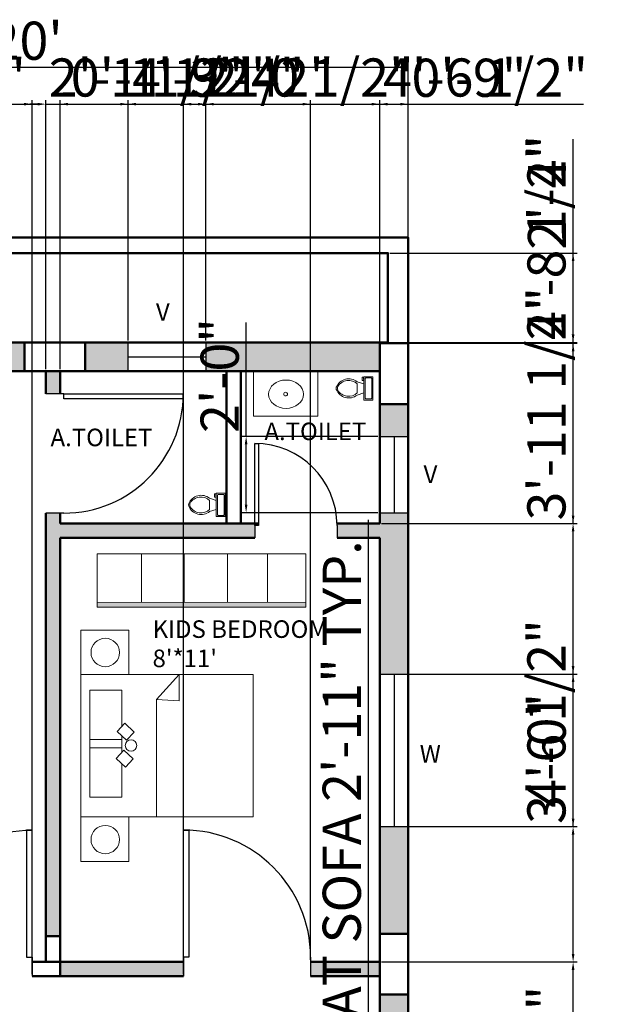
# Model space of a CAD drawing. Units: inches. Extents: x 2063 to 3370, y 2091 to 2971.
# Tile 14 of 14: x 3185 to 3370, y 2623 to 2933. Entities that reach past the tile are written whole.
import ezdxf

# ---------------------------------------------------------------- set-up
doc = ezdxf.new("R2010")
doc.units = ezdxf.units.IN
for name, color, linetype, lineweight in [('A-ANNO-DIMS', 2, 'Continuous', 18), ('A-ANNO-TEXT', 7, 'Continuous', 18), ('A-AREA-IDEN', 3, 'Continuous', 18), ('A-COLS', 7, 'Continuous', 50), ('A-DOOR', 4, 'Continuous', 25), ('A-FLOR-FIXT', 9, 'Continuous', 18), ('A-FURN', 8, 'Continuous', 18), ('A-GLAZ', 131, 'Continuous', 25), ('A-WALL', 7, 'Continuous', 50), ('A-WALL-PATT', 8, 'Continuous', 13)]:
    doc.layers.add(name, color=color, linetype=linetype, lineweight=lineweight)
doc.styles.get("Standard").update_dxf_attribs({"font": 'arial.ttf'})
doc.dimstyles.new('ISO-25', dxfattribs={"dimtxt": 12, "dimasz": 2.5, "dimexe": 1.25, "dimexo": 0.625, "dimtad": 1, "dimdec": 0, "dimlunit": 4, "dimtxsty": 'Standard', "dimcen": 2.5, "dimadec": 0, "dimazin": 0, "dimtfac": 1, "dimtdec": 0, "dimtmove": 0, "dimatfit": 3, "dimfxl": 1, "dimarcsym": 0})

# ---------------------------------------------------------------- blocks, each defined once
blk = doc.blocks.new('*U2')
for p, q in [((0, 0), (0, -6)), ((40, 0), (40, -6))]:
    blk.add_line(p, q)
blk.add_lwpolyline([(0, 0), (0, 40), (1.75, 40), (1.75, 0)], close=True)
blk.add_arc((0, 0), 40, 0, 90)
blk = doc.blocks.new('*U4')
for p, q in [((-10, -8.5), (-8, -8.5)), ((-10, -9.5), (-10, -8.5)), ((-8, -8.5), (-8, -8)), ((-7, -8), (-7, -9.5)), ((-4, -8), (-6, -14)), ((4, -8), (6, -14)), ((9.5, -6), (9.5, -2)), ((-7, -9.5), (-10, -9.5)), ((4, -14), (-4, -14))]:
    blk.add_line(p, q)
blk.add_lwpolyline([(10.5, -8), (10.5, 0), (-10.5, 0), (-10.5, -8)], close=True)
for points in [[(-9.5, -2), (-9.5, -6)], [(8.5, -1), (-8.5, -1)], [(-8.5, -7), (8.5, -7)]]:
    blk.add_lwpolyline(points)
for centre, radius, start, end in [((-8.62, -1.88), 0.884, 81.8699, 188.1301), ((-8.62, -6.12), 0.884, 171.8699, 278.1301), ((8.62, -1.88), 0.884, 351.8699, 98.1301), ((8.62, -6.12), 0.884, 261.8699, 8.1301), ((3.52, -21.58), 12.17, 141.46911, 247.97143), ((4.2, -21.82), 11.33, 136.36773, 238.94682), ((-3.52, -21.58), 12.17, 292.02843, 38.53071), ((-4.2, -21.82), 11.33, 301.05301, 43.63209), ((0, -27.88), 4, 245.73182, 294.26817), ((0, -29), 4, 254.86053, 285.13947)]:
    blk.add_arc(centre, radius, start, end)
blk = doc.blocks.new('*D9')
at = {"layer": 'A-ANNO-DIMS', "color": 0, "lineweight": -2, "transparency": 16777216}
for p, q in [((3067.42, 2865.05), (3067.42, 2919.33)), ((3069.92, 2918.08), (3304.92, 2918.08)), ((3307.42, 2865.05), (3307.42, 2919.33))]:
    blk.add_line(p, q, dxfattribs=at)
at = {"layer": 'A-ANNO-DIMS', "color": 0, "transparency": 16777216}
for points in [[(3069.92, 2918.5), (3069.92, 2917.67), (3067.42, 2918.08)], [(3304.92, 2918.5), (3304.92, 2917.67), (3307.42, 2918.08)]]:
    blk.add_solid(points, dxfattribs=at)
at = {"layer": 'Defpoints', "color": 0, "transparency": 16777216}
for p in [(3307.42, 2918.08), (3067.42, 2864.43), (3307.42, 2864.43)]:
    blk.add_point(p, dxfattribs=at)
at = {"layer": 'A-ANNO-DIMS', "color": 0, "transparency": 16777216, "insert": (3187.42, 2924.84), "char_height": 12, "attachment_point": 5}
blk.add_mtext("20'", dxfattribs=at)
blk = doc.blocks.new('BED-DOUBLE')
for p, q in [((23.79, 50.98), (30.96, 58.78)), ((30.96, 58.78), (30.96, 50.54)), ((23.79, 14), (23.79, 50.98)), ((30.96, 50.54), (23.79, 50.98))]:
    blk.add_line(p, q)
for points in [[(0, 58.78), (15.11, 58.78), (15.11, 72.78), (0, 72.78)], [(0, 58.78), (54.26, 58.78), (54.26, 14), (0, 14)], [(11.45, 40.86), (13.89, 43.46), (16.84, 40.71), (14.4, 38.1)], [(11.16, 32.43), (13.59, 35.03), (16.54, 32.28), (14.11, 29.67)], [(0, 0), (15.11, 0), (15.11, 14), (0, 14)]]:
    blk.add_lwpolyline(points, close=True)
for points in [[(12.88, 42.39), (12.88, 53.87), (2.9, 53.87), (2.9, 35.71), (12.88, 35.71), (12.88, 39.52)], [(12.88, 34.27), (12.88, 38.39), (2.9, 38.39), (2.9, 20.23), (12.88, 20.23), (12.88, 30.81)]]:
    blk.add_lwpolyline(points)
for centre, radius in [((7.71, 65.74), 4.47), ((15.81, 36.46), 1.81), ((7.71, 6.86), 4.47)]:
    blk.add_circle(centre, radius)
blk = doc.blocks.new('WARDROBE')
for p, q in [((13.88, 1.44), (13.88, 16.75)), ((27.33, 1.44), (27.33, 16.75)), ((40.97, 1.44), (40.97, 16.75)), ((53.56, 1.44), (53.56, 16.75)), ((0, 1.42), (65.55, 1.52))]:
    blk.add_line(p, q)
blk.add_lwpolyline([(0, 16.75), (65.55, 16.75), (65.55, 0), (0, 0)], close=True)
blk = doc.blocks.new('*D26')
at = {"layer": 'A-ANNO-DIMS', "color": 0, "lineweight": -2, "transparency": 16777216}
for p, q in [((3294.89, 2575.71), (3294.89, 2775.57)), ((3290.25, 2575.71), (3296.14, 2575.71)), ((3294.89, 2543.09), (3294.89, 2573.21)), ((3290.25, 2540.59), (3296.14, 2540.59))]:
    blk.add_line(p, q, dxfattribs=at)
at = {"layer": 'A-ANNO-DIMS', "color": 0, "transparency": 16777216}
for points in [[(3294.47, 2573.21), (3295.31, 2573.21), (3294.89, 2575.71)], [(3294.47, 2543.09), (3295.31, 2543.09), (3294.89, 2540.59)]]:
    blk.add_solid(points, dxfattribs=at)
at = {"layer": 'Defpoints', "color": 0, "transparency": 16777216}
for p in [(3289.62, 2575.71), (3294.89, 2575.71), (3289.62, 2540.59)]:
    blk.add_point(p, dxfattribs=at)
at = {"layer": 'A-ANNO-DIMS', "color": 0, "transparency": 16777216, "insert": (3288.05, 2676.89), "char_height": 12, "attachment_point": 5, "rotation": 90}
blk.add_mtext('3-SEAT SOFA 2\'-11" TYP.', dxfattribs=at)
blk = doc.blocks.new('*D138')
at = {"layer": 'A-ANNO-DIMS', "color": 0, "lineweight": -2, "transparency": 16777216}
for p, q in [((3167.94, 2832.05), (3167.94, 2907.68)), ((3193.42, 2823.05), (3193.42, 2907.68)), ((3170.44, 2906.43), (3190.92, 2906.43)), ((3193.42, 2906.43), (3257.23, 2906.43))]:
    blk.add_line(p, q, dxfattribs=at)
at = {"layer": 'A-ANNO-DIMS', "color": 0, "transparency": 16777216}
for points in [[(3170.44, 2906.84), (3170.44, 2906.01), (3167.94, 2906.43)], [(3190.92, 2906.84), (3190.92, 2906.01), (3193.42, 2906.43)]]:
    blk.add_solid(points, dxfattribs=at)
at = {"layer": 'Defpoints', "color": 0, "transparency": 16777216}
for p in [(3193.42, 2906.43), (3167.94, 2831.43), (3193.42, 2822.43)]:
    blk.add_point(p, dxfattribs=at)
at = {"layer": 'A-ANNO-DIMS', "color": 0, "transparency": 16777216, "insert": (3226.57, 2913.26), "char_height": 12, "attachment_point": 5}
blk.add_mtext('2\'-1 1/2"', dxfattribs=at)
blk = doc.blocks.new('*D139')
at = {"layer": 'A-ANNO-DIMS', "color": 0, "lineweight": -2, "transparency": 16777216}
for p, q in [((3193.42, 2823.05), (3193.42, 2907.68)), ((3197.92, 2823.05), (3197.92, 2907.68)), ((3190.92, 2906.43), (3188.42, 2906.43)), ((3193.42, 2906.43), (3197.92, 2906.43)), ((3200.42, 2906.43), (3264.03, 2906.43))]:
    blk.add_line(p, q, dxfattribs=at)
at = {"layer": 'A-ANNO-DIMS', "color": 0, "transparency": 16777216}
for points in [[(3190.92, 2906.84), (3190.92, 2906.01), (3193.42, 2906.43)], [(3200.42, 2906.84), (3200.42, 2906.01), (3197.92, 2906.43)]]:
    blk.add_solid(points, dxfattribs=at)
at = {"layer": 'Defpoints', "color": 0, "transparency": 16777216}
for p in [(3197.92, 2906.43), (3193.42, 2822.43), (3197.92, 2822.43)]:
    blk.add_point(p, dxfattribs=at)
at = {"layer": 'A-ANNO-DIMS', "color": 0, "transparency": 16777216, "insert": (3233.47, 2913.26), "char_height": 12, "attachment_point": 5}
blk.add_mtext('0\'-4 1/2"', dxfattribs=at)
blk = doc.blocks.new('*D140')
at = {"layer": 'A-ANNO-DIMS', "color": 0, "lineweight": -2, "transparency": 16777216}
for p, q in [((3197.92, 2823.05), (3197.92, 2907.68)), ((3219.33, 2832.05), (3219.33, 2907.68)), ((3200.42, 2906.43), (3216.83, 2906.43)), ((3219.33, 2906.43), (3281.81, 2906.43))]:
    blk.add_line(p, q, dxfattribs=at)
at = {"layer": 'A-ANNO-DIMS', "color": 0, "transparency": 16777216}
for points in [[(3200.42, 2906.84), (3200.42, 2906.01), (3197.92, 2906.43)], [(3216.83, 2906.84), (3216.83, 2906.01), (3219.33, 2906.43)]]:
    blk.add_solid(points, dxfattribs=at)
at = {"layer": 'Defpoints', "color": 0, "transparency": 16777216}
for p in [(3219.33, 2906.43), (3219.33, 2831.43), (3197.92, 2822.43)]:
    blk.add_point(p, dxfattribs=at)
at = {"layer": 'A-ANNO-DIMS', "color": 0, "transparency": 16777216, "insert": (3251.82, 2913.26), "char_height": 12, "attachment_point": 5}
blk.add_mtext('1\'-9 1/2"', dxfattribs=at)
blk = doc.blocks.new('*D141')
at = {"layer": 'A-ANNO-DIMS', "color": 0, "lineweight": -2, "transparency": 16777216}
for p, q in [((3219.33, 2832.05), (3219.33, 2907.68)), ((3243.76, 2832.05), (3243.76, 2907.68)), ((3221.83, 2906.43), (3241.26, 2906.43)), ((3243.76, 2906.43), (3307.58, 2906.43))]:
    blk.add_line(p, q, dxfattribs=at)
at = {"layer": 'A-ANNO-DIMS', "color": 0, "transparency": 16777216}
for points in [[(3221.83, 2906.84), (3221.83, 2906.01), (3219.33, 2906.43)], [(3241.26, 2906.84), (3241.26, 2906.01), (3243.76, 2906.43)]]:
    blk.add_solid(points, dxfattribs=at)
at = {"layer": 'Defpoints', "color": 0, "transparency": 16777216}
for p in [(3243.76, 2906.43), (3219.33, 2831.43), (3243.76, 2831.43)]:
    blk.add_point(p, dxfattribs=at)
at = {"layer": 'A-ANNO-DIMS', "color": 0, "transparency": 16777216, "insert": (3276.92, 2913.26), "char_height": 12, "attachment_point": 5}
blk.add_mtext('2\'-0 1/2"', dxfattribs=at)
blk = doc.blocks.new('*D142')
at = {"layer": 'A-ANNO-DIMS', "color": 0, "lineweight": -2, "transparency": 16777216}
for p, q in [((3243.76, 2832.05), (3243.76, 2907.68)), ((3298.42, 2823.05), (3298.42, 2907.68)), ((3246.26, 2906.43), (3295.92, 2906.43)), ((3298.42, 2906.43), (3362.51, 2906.43))]:
    blk.add_line(p, q, dxfattribs=at)
at = {"layer": 'A-ANNO-DIMS', "color": 0, "transparency": 16777216}
for points in [[(3246.26, 2906.84), (3246.26, 2906.01), (3243.76, 2906.43)], [(3295.92, 2906.84), (3295.92, 2906.01), (3298.42, 2906.43)]]:
    blk.add_solid(points, dxfattribs=at)
at = {"layer": 'Defpoints', "color": 0, "transparency": 16777216}
for p in [(3298.42, 2906.43), (3243.76, 2831.43), (3298.42, 2822.43)]:
    blk.add_point(p, dxfattribs=at)
at = {"layer": 'A-ANNO-DIMS', "color": 0, "transparency": 16777216, "insert": (3331.71, 2913.26), "char_height": 12, "attachment_point": 5}
blk.add_mtext('4\'-6 1/2"', dxfattribs=at)
blk = doc.blocks.new('*D143')
at = {"layer": 'A-ANNO-DIMS', "color": 0, "lineweight": -2, "transparency": 16777216}
for p, q in [((3298.42, 2823.05), (3298.42, 2907.68)), ((3307.42, 2831.77), (3307.42, 2907.68)), ((3300.92, 2906.43), (3304.92, 2906.43)), ((3307.42, 2906.43), (3343.06, 2906.43))]:
    blk.add_line(p, q, dxfattribs=at)
at = {"layer": 'A-ANNO-DIMS', "color": 0, "transparency": 16777216}
for points in [[(3300.92, 2906.84), (3300.92, 2906.01), (3298.42, 2906.43)], [(3304.92, 2906.84), (3304.92, 2906.01), (3307.42, 2906.43)]]:
    blk.add_solid(points, dxfattribs=at)
at = {"layer": 'Defpoints', "color": 0, "transparency": 16777216}
for p in [(3307.42, 2906.43), (3307.42, 2831.15), (3298.42, 2822.43)]:
    blk.add_point(p, dxfattribs=at)
at = {"layer": 'A-ANNO-DIMS', "color": 0, "transparency": 16777216, "insert": (3326.49, 2913.18), "char_height": 12, "attachment_point": 5}
blk.add_mtext('0\'-9"', dxfattribs=at)
blk = doc.blocks.new('*D164')
at = {"layer": 'A-ANNO-DIMS', "color": 0, "lineweight": -2, "transparency": 16777216}
for p, q in [((3299.04, 2636.43), (3360.49, 2636.43)), ((3359.24, 2587.78), (3359.24, 2633.93)), ((3299.04, 2585.28), (3360.49, 2585.28))]:
    blk.add_line(p, q, dxfattribs=at)
at = {"layer": 'A-ANNO-DIMS', "color": 0, "transparency": 16777216}
for points in [[(3358.82, 2633.93), (3359.66, 2633.93), (3359.24, 2636.43)], [(3358.82, 2587.78), (3359.66, 2587.78), (3359.24, 2585.28)]]:
    blk.add_solid(points, dxfattribs=at)
at = {"layer": 'Defpoints', "color": 0, "transparency": 16777216}
for p in [(3298.42, 2636.43), (3359.24, 2636.43), (3298.42, 2585.28)]:
    blk.add_point(p, dxfattribs=at)
at = {"layer": 'A-ANNO-DIMS', "color": 0, "transparency": 16777216, "insert": (3352.48, 2610.85), "char_height": 12, "attachment_point": 5, "rotation": 90}
blk.add_mtext('4\'-3"', dxfattribs=at)
blk = doc.blocks.new('*D165')
at = {"layer": 'A-ANNO-DIMS', "color": 0, "lineweight": -2, "transparency": 16777216}
for p, q in [((3359.24, 2679.03), (3359.24, 2742.63)), ((3299.04, 2679.03), (3360.49, 2679.03)), ((3359.24, 2638.93), (3359.24, 2676.53)), ((3299.04, 2636.43), (3360.49, 2636.43))]:
    blk.add_line(p, q, dxfattribs=at)
at = {"layer": 'A-ANNO-DIMS', "color": 0, "transparency": 16777216}
for points in [[(3358.82, 2676.53), (3359.66, 2676.53), (3359.24, 2679.03)], [(3358.82, 2638.93), (3359.66, 2638.93), (3359.24, 2636.43)]]:
    blk.add_solid(points, dxfattribs=at)
at = {"layer": 'Defpoints', "color": 0, "transparency": 16777216}
for p in [(3298.42, 2679.03), (3359.24, 2679.03), (3298.42, 2636.43)]:
    blk.add_point(p, dxfattribs=at)
at = {"layer": 'A-ANNO-DIMS', "color": 0, "transparency": 16777216, "insert": (3352.41, 2712.08), "char_height": 12, "attachment_point": 5, "rotation": 90}
blk.add_mtext('3\'-6 1/2"', dxfattribs=at)
blk = doc.blocks.new('*D166')
at = {"layer": 'A-ANNO-DIMS', "color": 0, "lineweight": -2, "transparency": 16777216}
for p, q in [((3299.04, 2727.03), (3360.49, 2727.03)), ((3359.24, 2681.53), (3359.24, 2724.53)), ((3299.04, 2679.03), (3360.49, 2679.03))]:
    blk.add_line(p, q, dxfattribs=at)
at = {"layer": 'A-ANNO-DIMS', "color": 0, "transparency": 16777216}
for points in [[(3358.82, 2724.53), (3359.66, 2724.53), (3359.24, 2727.03)], [(3358.82, 2681.53), (3359.66, 2681.53), (3359.24, 2679.03)]]:
    blk.add_solid(points, dxfattribs=at)
at = {"layer": 'Defpoints', "color": 0, "transparency": 16777216}
for p in [(3298.42, 2727.03), (3359.24, 2727.03), (3298.42, 2679.03)]:
    blk.add_point(p, dxfattribs=at)
at = {"layer": 'A-ANNO-DIMS', "color": 0, "transparency": 16777216, "insert": (3352.49, 2703.03), "char_height": 12, "attachment_point": 5, "rotation": 90}
blk.add_mtext('4\'-0"', dxfattribs=at)
blk = doc.blocks.new('*D167')
at = {"layer": 'A-ANNO-DIMS', "color": 0, "lineweight": -2, "transparency": 16777216}
for p, q in [((3359.24, 2774.43), (3359.24, 2847.35)), ((3299.04, 2774.43), (3360.49, 2774.43)), ((3359.24, 2729.53), (3359.24, 2771.93)), ((3299.04, 2727.03), (3360.49, 2727.03))]:
    blk.add_line(p, q, dxfattribs=at)
at = {"layer": 'A-ANNO-DIMS', "color": 0, "transparency": 16777216}
for points in [[(3358.82, 2771.93), (3359.66, 2771.93), (3359.24, 2774.43)], [(3358.82, 2729.53), (3359.66, 2729.53), (3359.24, 2727.03)]]:
    blk.add_solid(points, dxfattribs=at)
at = {"layer": 'Defpoints', "color": 0, "transparency": 16777216}
for p in [(3298.42, 2774.43), (3359.24, 2774.43), (3298.42, 2727.03)]:
    blk.add_point(p, dxfattribs=at)
at = {"layer": 'A-ANNO-DIMS', "color": 0, "transparency": 16777216, "insert": (3352.41, 2812.14), "char_height": 12, "attachment_point": 5, "rotation": 90}
blk.add_mtext('3\'-11 1/2"', dxfattribs=at)
blk = doc.blocks.new('*D168')
at = {"layer": 'A-ANNO-DIMS', "color": 0, "lineweight": -2, "transparency": 16777216}
for p, q in [((3359.24, 2831.15), (3359.24, 2895.24)), ((3299.04, 2831.15), (3360.49, 2831.15)), ((3359.24, 2776.93), (3359.24, 2828.65)), ((3299.04, 2774.43), (3360.49, 2774.43))]:
    blk.add_line(p, q, dxfattribs=at)
at = {"layer": 'A-ANNO-DIMS', "color": 0, "transparency": 16777216}
for points in [[(3358.82, 2828.65), (3359.66, 2828.65), (3359.24, 2831.15)], [(3358.82, 2776.93), (3359.66, 2776.93), (3359.24, 2774.43)]]:
    blk.add_solid(points, dxfattribs=at)
at = {"layer": 'Defpoints', "color": 0, "transparency": 16777216}
for p in [(3298.42, 2831.15), (3359.24, 2831.15), (3298.42, 2774.43)]:
    blk.add_point(p, dxfattribs=at)
at = {"layer": 'A-ANNO-DIMS', "color": 0, "transparency": 16777216, "insert": (3352.41, 2864.44), "char_height": 12, "attachment_point": 5, "rotation": 90}
blk.add_mtext('4\'-8 1/2"', dxfattribs=at)
blk = doc.blocks.new('*D169')
at = {"layer": 'A-ANNO-DIMS', "color": 0, "lineweight": -2, "transparency": 16777216}
for p, q in [((3359.24, 2859.54), (3359.24, 2895.4)), ((3301.66, 2859.54), (3360.49, 2859.54)), ((3359.24, 2833.93), (3359.24, 2857.04)), ((3301.66, 2831.43), (3360.49, 2831.43))]:
    blk.add_line(p, q, dxfattribs=at)
at = {"layer": 'A-ANNO-DIMS', "color": 0, "transparency": 16777216}
for points in [[(3358.82, 2857.04), (3359.66, 2857.04), (3359.24, 2859.54)], [(3358.82, 2833.93), (3359.66, 2833.93), (3359.24, 2831.43)]]:
    blk.add_solid(points, dxfattribs=at)
at = {"layer": 'Defpoints', "color": 0, "transparency": 16777216}
for p in [(3301.03, 2859.54), (3359.24, 2859.54), (3301.03, 2831.43)]:
    blk.add_point(p, dxfattribs=at)
at = {"layer": 'A-ANNO-DIMS', "color": 0, "transparency": 16777216, "insert": (3352.59, 2878.72), "char_height": 12, "attachment_point": 5, "rotation": 90}
blk.add_mtext('2\'-4"', dxfattribs=at)
blk = doc.blocks.new('*D170')
at = {"layer": 'A-ANNO-DIMS', "color": 0, "lineweight": -2, "transparency": 16777216}
for p, q in [((3256.42, 2801.84), (3256.42, 2837.7)), ((3297.79, 2801.84), (3255.17, 2801.84)), ((3256.42, 2780.34), (3256.42, 2799.34)), ((3297.79, 2777.84), (3255.17, 2777.84))]:
    blk.add_line(p, q, dxfattribs=at)
at = {"layer": 'A-ANNO-DIMS', "color": 0, "transparency": 16777216}
for points in [[(3256, 2799.34), (3256.83, 2799.34), (3256.42, 2801.84)], [(3256, 2780.34), (3256.83, 2780.34), (3256.42, 2777.84)]]:
    blk.add_solid(points, dxfattribs=at)
at = {"layer": 'Defpoints', "color": 0, "transparency": 16777216}
for p in [(3256.42, 2801.84), (3298.42, 2801.84), (3298.42, 2777.84)]:
    blk.add_point(p, dxfattribs=at)
at = {"layer": 'A-ANNO-DIMS', "color": 0, "transparency": 16777216, "insert": (3249.66, 2821.02), "char_height": 12, "attachment_point": 5, "rotation": 90}
blk.add_mtext('2\'-0"', dxfattribs=at)
blk = doc.blocks.new('*D173')
at = {"layer": 'A-ANNO-DIMS', "color": 0, "lineweight": -2, "transparency": 16777216}
for p, q in [((3149.1, 2637.05), (3149.1, 2907.68)), ((3189.1, 2632.55), (3189.1, 2907.68)), ((3151.6, 2906.43), (3186.6, 2906.43))]:
    blk.add_line(p, q, dxfattribs=at)
at = {"layer": 'A-ANNO-DIMS', "color": 0, "transparency": 16777216}
for points in [[(3151.6, 2906.84), (3151.6, 2906.01), (3149.1, 2906.43)], [(3186.6, 2906.84), (3186.6, 2906.01), (3189.1, 2906.43)]]:
    blk.add_solid(points, dxfattribs=at)
at = {"layer": 'Defpoints', "color": 0, "transparency": 16777216}
for p in [(3189.1, 2906.43), (3149.1, 2636.43), (3189.1, 2631.93)]:
    blk.add_point(p, dxfattribs=at)
at = {"layer": 'A-ANNO-DIMS', "color": 0, "transparency": 16777216, "insert": (3169.1, 2913.18), "char_height": 12, "attachment_point": 5}
blk.add_mtext('3\'-4"', dxfattribs=at)
blk = doc.blocks.new('*D174')
at = {"layer": 'A-ANNO-DIMS', "color": 0, "lineweight": -2, "transparency": 16777216}
for p, q in [((3236.69, 2632.55), (3236.69, 2907.68)), ((3276.69, 2637.05), (3276.69, 2907.68)), ((3239.19, 2906.43), (3274.19, 2906.43))]:
    blk.add_line(p, q, dxfattribs=at)
at = {"layer": 'A-ANNO-DIMS', "color": 0, "transparency": 16777216}
for points in [[(3239.19, 2906.84), (3239.19, 2906.01), (3236.69, 2906.43)], [(3274.19, 2906.84), (3274.19, 2906.01), (3276.69, 2906.43)]]:
    blk.add_solid(points, dxfattribs=at)
at = {"layer": 'Defpoints', "color": 0, "transparency": 16777216}
for p in [(3276.69, 2906.43), (3276.69, 2636.43), (3236.69, 2631.93)]:
    blk.add_point(p, dxfattribs=at)
at = {"layer": 'A-ANNO-DIMS', "color": 0, "transparency": 16777216, "insert": (3256.69, 2913.18), "char_height": 12, "attachment_point": 5}
blk.add_mtext('3\'-4"', dxfattribs=at)

msp = doc.modelspace()

# ---------------------------------------------------------------- hatches: boundary and pattern name
at = {"layer": 'A-FURN'}
h = msp.add_hatch(color=256, dxfattribs=at)
h.dxf.hatch_style = 1
h.paths.add_polyline_path([(3275.16, 2749.65), (3209.62, 2749.56), (3209.62, 2748.13), (3275.16, 2748.13)])
at = {"layer": 'A-WALL-PATT'}
h = msp.add_hatch(color=256, dxfattribs=at)
h.dxf.hatch_style = 1
h.paths.add_polyline_path([(3181.8, 2234.43), (3076.42, 2234.43), (3076.42, 2232.93), (3076.42, 2225.43), (3181.8, 2225.43)])
h.paths.add_polyline_path([(3212.92, 2192.43), (3200.92, 2192.43), (3104.92, 2192.43), (3104.92, 2189.43), (3104.92, 2187.43), (3200.92, 2187.43), (3212.92, 2187.42)], flags=17)
h.paths.add_polyline_path([(3219.45, 2153.43), (3076.42, 2153.43), (3076.42, 2222.57), (3067.42, 2222.57), (3067.42, 2144.43), (3219.45, 2144.43)])
h.paths.add_polyline_path([(3076.42, 2343.93), (3076.42, 2351.28), (3067.42, 2351.28), (3067.42, 2241.68), (3076.42, 2241.68), (3076.42, 2258.43)])
h.paths.add_polyline_path([(3175.73, 2554.94), (3230.21, 2554.94), (3230.21, 2575.54), (3175.73, 2575.54)], flags=9)
h.paths.add_polyline_path([(3085.27, 2530.92), (3121.9, 2530.92), (3121.9, 2551.53), (3085.27, 2551.53)], flags=9)
h.paths.add_polyline_path([(3089.9, 2596.23), (3114.49, 2596.23), (3114.49, 2616.83), (3089.9, 2616.83)], flags=9)
h.paths.add_polyline_path([(3260.79, 2797.55), (3297.86, 2797.55), (3297.86, 2808.94), (3260.79, 2808.94)], flags=9)
h.paths.add_polyline_path([(3113.05, 2696.74), (3189.97, 2696.74), (3189.97, 2717.35), (3113.05, 2717.35)], flags=9)
h.paths.add_polyline_path([(3226.64, 2835.24), (3234.55, 2835.24), (3234.55, 2846.62), (3226.64, 2846.62)], flags=9)
h.paths.add_polyline_path([(3140.56, 2833.68), (3150.6, 2833.68), (3150.6, 2845.06), (3140.56, 2845.06)], flags=9)
h.paths.add_polyline_path([(3193.53, 2795.64), (3230.6, 2795.64), (3230.6, 2807.02), (3193.53, 2807.02)], flags=9)
h.paths.add_polyline_path([(3225.05, 2726.09), (3287.83, 2726.09), (3287.83, 2746.7), (3225.05, 2746.7)], flags=9)
h = msp.add_hatch(color=256, dxfattribs=at)
h.dxf.hatch_style = 1
h.paths.add_polyline_path([(3294.05, 2153.43), (3219.45, 2153.43), (3219.45, 2144.43), (3294.05, 2144.43)])
h.paths.add_polyline_path([(3307.42, 2220.3), (3298.42, 2220.3), (3298.42, 2153.43), (3294.05, 2153.43), (3294.05, 2144.43), (3307.42, 2144.43)])
h.paths.add_polyline_path([(3076.42, 2468.43), (3076.42, 2477.43), (3076.42, 2514.15), (3067.42, 2514.15), (3067.42, 2370.39), (3076.42, 2370.39)])
h.paths.add_polyline_path([(3307.42, 2525.28), (3298.42, 2525.28), (3298.42, 2523.93), (3298.42, 2466.93), (3298.42, 2383.04), (3307.42, 2383.04)])
h.paths.add_polyline_path([(3307.42, 2363.93), (3298.42, 2363.93), (3298.42, 2239.41), (3307.42, 2239.41)])
h.paths.add_polyline_path([(3235.32, 2180.53), (3274.95, 2180.53), (3274.95, 2201.14), (3235.32, 2201.14)], flags=9)
h.paths.add_polyline_path([(3127.74, 2323.36), (3191.84, 2323.36), (3191.84, 2343.96), (3127.74, 2343.96)], flags=9)
h.paths.add_polyline_path([(3175.73, 2554.94), (3230.21, 2554.94), (3230.21, 2575.54), (3175.73, 2575.54)], flags=9)
h.paths.add_polyline_path([(3085.27, 2530.92), (3121.9, 2530.92), (3121.9, 2551.53), (3085.27, 2551.53)], flags=9)
h.paths.add_polyline_path([(3089.9, 2596.23), (3114.49, 2596.23), (3114.49, 2616.83), (3089.9, 2616.83)], flags=9)
h.paths.add_polyline_path([(3260.79, 2797.55), (3297.86, 2797.55), (3297.86, 2808.94), (3260.79, 2808.94)], flags=9)
h.paths.add_polyline_path([(3113.05, 2696.74), (3189.97, 2696.74), (3189.97, 2717.35), (3113.05, 2717.35)], flags=9)
h.paths.add_polyline_path([(3226.64, 2835.24), (3234.55, 2835.24), (3234.55, 2846.62), (3226.64, 2846.62)], flags=9)
h.paths.add_polyline_path([(3140.56, 2833.68), (3150.6, 2833.68), (3150.6, 2845.06), (3140.56, 2845.06)], flags=9)
h.paths.add_polyline_path([(3193.53, 2795.64), (3230.6, 2795.64), (3230.6, 2807.02), (3193.53, 2807.02)], flags=9)
h.paths.add_polyline_path([(3225.05, 2726.09), (3287.83, 2726.09), (3287.83, 2746.7), (3225.05, 2746.7)], flags=9)
h = msp.add_hatch(color=256, dxfattribs=at)
h.dxf.hatch_style = 1
h.paths.add_polyline_path([(3076.42, 2619.52), (3067.42, 2619.52), (3067.42, 2548.5), (3076.42, 2548.5), (3076.42, 2579.43)])
h.paths.add_polyline_path([(3236.69, 2636.43), (3197.92, 2636.43), (3197.92, 2631.93), (3236.69, 2631.93)])
h.paths.add_polyline_path([(3145.42, 2631.93), (3149.1, 2631.93), (3149.1, 2636.43), (3147.77, 2636.43), (3076.42, 2636.43), (3076.42, 2631.93), (3113.39, 2631.93), (3136.42, 2631.93), (3140.92, 2631.93), (3140.92, 2623.58), (3142.89, 2623.58), (3145.42, 2623.58)])
h.paths.add_polyline_path([(3298.42, 2636.43), (3276.69, 2636.43), (3276.69, 2631.93), (3298.42, 2631.93)])
h.paths.add_polyline_path([(3307.42, 2679.03), (3298.42, 2679.03), (3298.42, 2645.28), (3307.42, 2645.28)])
h.paths.add_polyline_path([(3307.42, 2626.16), (3298.42, 2626.16), (3298.42, 2585.28), (3307.42, 2585.28)])
h.paths.add_polyline_path([(3260.79, 2797.55), (3297.86, 2797.55), (3297.86, 2808.94), (3260.79, 2808.94)], flags=9)
h.paths.add_polyline_path([(3113.05, 2696.74), (3189.97, 2696.74), (3189.97, 2717.35), (3113.05, 2717.35)], flags=9)
h.paths.add_polyline_path([(3226.64, 2835.24), (3234.55, 2835.24), (3234.55, 2846.62), (3226.64, 2846.62)], flags=9)
h.paths.add_polyline_path([(3140.56, 2833.68), (3150.6, 2833.68), (3150.6, 2845.06), (3140.56, 2845.06)], flags=9)
h.paths.add_polyline_path([(3193.53, 2795.64), (3230.6, 2795.64), (3230.6, 2807.02), (3193.53, 2807.02)], flags=9)
h.paths.add_polyline_path([(3225.05, 2726.09), (3287.83, 2726.09), (3287.83, 2746.7), (3225.05, 2746.7)], flags=9)
h = msp.add_hatch(color=256, dxfattribs=at)
h.dxf.hatch_style = 1
h.paths.add_polyline_path([(3119.94, 2831.43), (3076.42, 2831.43), (3076.42, 2822.43), (3119.94, 2822.43)])
h.paths.add_polyline_path([(3186.73, 2831.43), (3167.94, 2831.43), (3167.94, 2822.43), (3186.73, 2822.43)])
h.paths.add_polyline_path([(3219.33, 2831.43), (3205.84, 2831.43), (3205.84, 2822.43), (3219.33, 2822.43)])
h.paths.add_polyline_path([(3298.42, 2831.43), (3243.76, 2831.43), (3243.76, 2822.43), (3298.42, 2822.43)])
h.paths.add_polyline_path([(3235.32, 2180.53), (3274.95, 2180.53), (3274.95, 2201.14), (3235.32, 2201.14)], flags=9)
h.paths.add_polyline_path([(3127.74, 2323.36), (3191.84, 2323.36), (3191.84, 2343.96), (3127.74, 2343.96)], flags=9)
h.paths.add_polyline_path([(3175.73, 2554.94), (3230.21, 2554.94), (3230.21, 2575.54), (3175.73, 2575.54)], flags=9)
h.paths.add_polyline_path([(3085.27, 2530.92), (3121.9, 2530.92), (3121.9, 2551.53), (3085.27, 2551.53)], flags=9)
h.paths.add_polyline_path([(3089.9, 2596.23), (3114.49, 2596.23), (3114.49, 2616.83), (3089.9, 2616.83)], flags=9)
h.paths.add_polyline_path([(3113.05, 2696.74), (3189.97, 2696.74), (3189.97, 2717.35), (3113.05, 2717.35)], flags=9)
h.paths.add_polyline_path([(3193.53, 2795.64), (3230.6, 2795.64), (3230.6, 2807.02), (3193.53, 2807.02)], flags=9)
h.paths.add_polyline_path([(3225.05, 2726.09), (3287.83, 2726.09), (3287.83, 2746.7), (3225.05, 2746.7)], flags=9)
h = msp.add_hatch(color=256, dxfattribs=at)
h.dxf.hatch_style = 1
h.paths.add_polyline_path([(3197.92, 2822.43), (3193.42, 2822.43), (3193.42, 2815.29), (3197.92, 2815.29)])
h.paths.add_polyline_path([(3307.42, 2812.03), (3298.42, 2812.03), (3298.42, 2801.84), (3307.42, 2801.84)])
edge = h.paths.add_edge_path()
edge.add_arc((3259.18, 2773.8), 25.82, 0, 1.391)
edge.add_line((3284.99, 2774.43), (3298.42, 2774.43))
edge.add_line((3298.42, 2774.43), (3298.42, 2777.84))
edge.add_line((3298.42, 2777.84), (3307.42, 2777.84))
edge.add_line((3307.42, 2777.84), (3307.42, 2727.03))
edge.add_line((3307.42, 2727.03), (3298.42, 2727.03))
edge.add_line((3298.42, 2727.03), (3298.42, 2769.93))
edge.add_line((3298.42, 2769.93), (3285, 2769.93))
edge.add_line((3285, 2769.93), (3285, 2773.8))
h.paths.add_polyline_path([(3259.18, 2769.93), (3259.18, 2774.43), (3197.92, 2774.43), (3197.92, 2777.68), (3193.42, 2777.68), (3193.42, 2644.58), (3197.92, 2644.58), (3197.92, 2769.93)])
h = msp.add_hatch(color=256, dxfattribs=at)
h.dxf.hatch_style = 1
h.paths.add_polyline_path([(3254.4, 2477.43), (3145.42, 2477.43), (3145.42, 2579.43), (3145.42, 2589.96), (3142.89, 2589.96), (3140.92, 2589.96), (3140.92, 2583.93), (3131.92, 2583.93), (3076.42, 2583.93), (3076.42, 2579.43), (3136.42, 2579.43), (3140.92, 2579.43), (3140.92, 2477.43), (3076.42, 2477.43), (3076.42, 2468.43), (3193.42, 2468.43), (3254.4, 2468.43), (3254.4, 2471.41)])
h.paths.add_polyline_path([(3235.32, 2180.53), (3274.95, 2180.53), (3274.95, 2201.14), (3235.32, 2201.14)], flags=9)
h.paths.add_polyline_path([(3127.74, 2323.36), (3191.84, 2323.36), (3191.84, 2343.96), (3127.74, 2343.96)], flags=9)
h.paths.add_polyline_path([(3175.73, 2554.94), (3230.21, 2554.94), (3230.21, 2575.54), (3175.73, 2575.54)], flags=25)
h.paths.add_polyline_path([(3089.9, 2596.23), (3114.49, 2596.23), (3114.49, 2616.83), (3089.9, 2616.83)], flags=9)
h.paths.add_polyline_path([(3260.79, 2797.55), (3297.86, 2797.55), (3297.86, 2808.94), (3260.79, 2808.94)], flags=9)
h.paths.add_polyline_path([(3113.05, 2696.74), (3189.97, 2696.74), (3189.97, 2717.35), (3113.05, 2717.35)], flags=9)
h.paths.add_polyline_path([(3193.53, 2795.64), (3230.6, 2795.64), (3230.6, 2807.02), (3193.53, 2807.02)], flags=9)
h.paths.add_polyline_path([(3225.05, 2726.09), (3287.83, 2726.09), (3287.83, 2746.7), (3225.05, 2746.7)], flags=9)

# ---------------------------------------------------------------- linework, layer by layer
at = {"layer": 'A-COLS'}
for points in [[(3186.73, 2822.43), (3186.73, 2831.43), (3205.84, 2831.43), (3205.84, 2822.43)], [(3298.42, 2831.15), (3307.42, 2831.15), (3307.42, 2812.03), (3298.42, 2812.03)]]:
    msp.add_lwpolyline(points, close=True, dxfattribs=at)
msp.add_lwpolyline([(3298.42, 2636.43), (3298.42, 2645.28), (3307.42, 2645.28), (3307.42, 2626.16), (3298.42, 2626.16), (3298.42, 2631.93)], dxfattribs=at)
at = {"layer": 'A-FLOR-FIXT'}
msp.add_lwpolyline([(3258.71, 2808.22), (3278.99, 2808.22), (3278.99, 2822.43), (3258.71, 2822.43)], close=True, dxfattribs=at)
msp.add_circle((3268.83, 2815.16), 0.596, dxfattribs=at)
msp.add_ellipse((3268.96, 2815.13), major_axis=(5.46, 0), ratio=0.818182, dxfattribs=at)
at = {"layer": 'A-GLAZ'}
for p, q in [((3219.33, 2826.93), (3243.76, 2826.93)), ((3298.42, 2801.84), (3307.42, 2801.84)), ((3302.92, 2801.84), (3302.92, 2777.84)), ((3298.42, 2777.84), (3307.42, 2777.84)), ((3298.42, 2727.03), (3307.42, 2727.03)), ((3302.92, 2727.03), (3302.92, 2679.03)), ((3298.42, 2679.03), (3307.42, 2679.03))]:
    msp.add_line(p, q, dxfattribs=at)
msp.add_lwpolyline([(3219.33, 2831.43), (3243.76, 2831.43), (3243.76, 2822.43), (3219.33, 2822.43)], close=True, dxfattribs=at)
at = {"layer": 'A-WALL'}
for p, q in [((3076.42, 2822.43), (3193.42, 2822.43)), ((3076.42, 2822.43), (3193.42, 2822.43)), ((3193.42, 2822.43), (3193.42, 2815.29)), ((3197.92, 2822.43), (3298.42, 2822.43)), ((3197.92, 2822.43), (3197.92, 2815.29)), ((3197.92, 2822.43), (3197.92, 2815.29)), ((3250.24, 2822.43), (3250.24, 2774.43)), ((3254.74, 2822.43), (3254.74, 2774.43)), ((3193.42, 2777.68), (3193.42, 2636.43)), ((3197.92, 2777.68), (3197.92, 2774.43)), ((3197.92, 2777.68), (3197.92, 2774.43)), ((3197.92, 2774.43), (3260.31, 2774.43)), ((3284.99, 2774.43), (3298.42, 2774.43)), ((3293.92, 2774.43), (3298.42, 2774.43)), ((3197.92, 2769.93), (3197.92, 2631.93)), ((3197.92, 2769.93), (3259.18, 2769.93)), ((3285, 2769.93), (3298.42, 2769.93)), ((3189.1, 2636.43), (3236.69, 2636.43)), ((3276.69, 2636.43), (3298.42, 2636.43)), ((3189.1, 2631.93), (3236.69, 2631.93)), ((3276.69, 2631.93), (3298.42, 2631.93))]:
    msp.add_line(p, q, dxfattribs=at)
for points in [[(3067.42, 2144.43), (3307.42, 2144.43), (3307.42, 2864.43), (3067.42, 2864.43)], [(3301.03, 2831.43), (3301.03, 2859.54), (3073.29, 2859.54), (3073.29, 2831.43)]]:
    msp.add_lwpolyline(points, close=True, dxfattribs=at)
for points in [[(3298.42, 2774.43), (3298.42, 2822.43)], [(3298.42, 2576.43), (3298.42, 2769.93)], [(3193.42, 2644.58), (3197.92, 2644.58), (3197.92, 2631.93)]]:
    msp.add_lwpolyline(points, dxfattribs=at)

# ---------------------------------------------------------------- block references
at = {"layer": 'A-DOOR', "xscale": 0.9400530028669262, "yscale": 0.9400530028669262, "zscale": 0.9400530028669262, "rotation": 270}
msp.add_blockref('*U2', (3199.06, 2815.29), dxfattribs=at)
at = {"layer": 'A-DOOR', "xscale": 0.645531349072257, "yscale": 0.645531349072257, "zscale": 0.645531349072257}
msp.add_blockref('*U2', (3259.18, 2773.8), dxfattribs=at)
at = {"layer": 'A-DOOR', "xscale": -1}
msp.add_blockref('*U2', (3189.1, 2637.93), dxfattribs=at)
at = {"layer": 'A-DOOR'}
msp.add_blockref('*U2', (3236.69, 2637.93), dxfattribs=at)
at = {"layer": 'A-FLOR-FIXT', "xscale": 0.3494779928887701, "yscale": 0.3494779928887701, "zscale": 0.3494779928887701, "rotation": 270}
for p in [(3296.27, 2816.96), (3249.84, 2780.28)]:
    msp.add_blockref('*U4', p, dxfattribs=at)
at = {"layer": 'A-FURN'}
for name, p in [('WARDROBE', (3209.61, 2748.13)), ('BED-DOUBLE', (3204.41, 2668.08))]:
    msp.add_blockref(name, p, dxfattribs=at)

# ---------------------------------------------------------------- texts
at = {"layer": 'A-ANNO-TEXT', "char_height": 5.52, "attachment_point": 1}
for s, insert in [('V', (3228.06, 2843.78)), ('V', (3312.22, 2792.69)), ('W', (3311.02, 2704.68))]:
    msp.add_mtext_dynamic_manual_height_columns(s, width=106.0361, gutter_width=27.61, heights=[0], dxfattribs=dict(at, insert=insert))
at = {"layer": 'A-AREA-IDEN', "attachment_point": 1}
for s, insert, char_height in [('A.TOILET', (3262.18, 2806.19), 5.523), ('A.TOILET', (3194.92, 2804.28), 5.523), ("KIDS BEDROOM\\P8'*11'", (3227, 2743.95), 5.5229)]:
    msp.add_mtext_dynamic_manual_height_columns(s, width=106.0361, gutter_width=27.61, heights=[0], dxfattribs=dict(at, insert=insert, char_height=char_height))

# ---------------------------------------------------------------- dimensions: what is measured, and where the dimension line sits
at = {"layer": 'A-ANNO-DIMS'}
for base, p1, p2, override, picture, middle in [((3307.42, 2918.08), (3067.42, 2864.43), (3307.42, 2864.43), {"dimclrd": 0, "dimclre": 0, "dimclrt": 0}, '*D9', (3187.42, 2924.84)), ((3193.42, 2906.43), (3167.94, 2831.43), (3193.42, 2822.43), {"dimdec": 1, "dimlfac": 1, "dimrnd": 0, "dimzin": 1, "dimdsep": 46, "dimlunit": 4, "dimfrac": 2}, '*D138', (3226.57, 2913.26)), ((3197.92, 2906.43), (3193.42, 2822.43), (3197.92, 2822.43), {"dimdec": 1, "dimlfac": 1, "dimrnd": 0, "dimzin": 1, "dimdsep": 46, "dimlunit": 4, "dimfrac": 2}, '*D139', (3233.47, 2913.26)), ((3219.33, 2906.43), (3197.92, 2822.43), (3219.33, 2831.43), {"dimdec": 1, "dimlfac": 1, "dimrnd": 0, "dimzin": 1, "dimdsep": 46, "dimlunit": 4, "dimfrac": 2}, '*D140', (3251.82, 2913.26)), ((3243.76, 2906.43), (3219.33, 2831.43), (3243.76, 2831.43), {"dimdec": 1, "dimlfac": 1, "dimrnd": 0, "dimzin": 1, "dimdsep": 46, "dimlunit": 4, "dimfrac": 2}, '*D141', (3276.92, 2913.26)), ((3298.42, 2906.43), (3243.76, 2831.43), (3298.42, 2822.43), {"dimdec": 1, "dimlfac": 1, "dimrnd": 0, "dimzin": 1, "dimdsep": 46, "dimlunit": 4, "dimfrac": 2}, '*D142', (3331.71, 2913.26)), ((3189.1, 2906.43), (3149.1, 2636.43), (3189.1, 2631.93), {"dimdec": 1, "dimlfac": 1, "dimrnd": 0, "dimzin": 1, "dimdsep": 46, "dimlunit": 4, "dimfrac": 2}, '*D173', (3169.1, 2913.18)), ((3276.69, 2906.43), (3236.69, 2631.93), (3276.69, 2636.43), {"dimdec": 1, "dimlfac": 1, "dimrnd": 0, "dimzin": 1, "dimdsep": 46, "dimlunit": 4, "dimfrac": 2}, '*D174', (3256.69, 2913.18)), ((3307.42, 2906.43), (3298.42, 2822.43), (3307.42, 2831.15), {"dimdec": 1, "dimlfac": 1, "dimrnd": 0, "dimzin": 1, "dimdsep": 46, "dimlunit": 4, "dimfrac": 2}, '*D143', (3326.49, 2913.18))]:
    dim = msp.add_linear_dim(base=base, p1=p1, p2=p2, dimstyle='ISO-25', override=override, dxfattribs=at)
    dim.commit()
    dim.dimension.update_dxf_attribs({"geometry": picture, "text_midpoint": middle})
for base, p1, p2, picture, middle in [((3359.24, 2831.15), (3298.42, 2774.43), (3298.42, 2831.15), '*D168', (3352.41, 2864.44)), ((3359.24, 2859.54), (3301.03, 2831.43), (3301.03, 2859.54), '*D169', (3352.59, 2878.72)), ((3359.24, 2774.43), (3298.42, 2727.03), (3298.42, 2774.43), '*D167', (3352.41, 2812.14)), ((3256.42, 2801.84), (3298.42, 2777.84), (3298.42, 2801.84), '*D170', (3249.66, 2821.02)), ((3359.24, 2679.03), (3298.42, 2636.43), (3298.42, 2679.03), '*D165', (3352.41, 2712.08)), ((3359.24, 2727.03), (3298.42, 2679.03), (3298.42, 2727.03), '*D166', (3352.49, 2703.03)), ((3359.2401, 2636.4264), (3298.4159, 2585.2786), (3298.4159, 2636.4264), '*D164', (3352.4841, 2610.8525))]:
    dim = msp.add_linear_dim(base=base, p1=p1, p2=p2, angle=90, dimstyle='ISO-25', override={"dimdec": 1, "dimlfac": 1, "dimrnd": 0, "dimzin": 1, "dimdsep": 46, "dimlunit": 4, "dimfrac": 2}, dxfattribs=at)
    dim.commit()
    dim.dimension.update_dxf_attribs({"geometry": picture, "text_midpoint": middle})
dim = msp.add_linear_dim(base=(3294.89, 2575.71), p1=(3289.62, 2540.59), p2=(3289.62, 2575.71), angle=90, text='3-SEAT SOFA <> TYP.', dimstyle='ISO-25', override={"dimdec": 1, "dimrnd": 0, "dimzin": 1, "dimlunit": 4, "dimfrac": 2}, dxfattribs=at)
dim.commit()
dim.dimension.update_dxf_attribs({"geometry": '*D26', "text_midpoint": (3288.05, 2676.89)})

doc.saveas('drawing.dxf')
